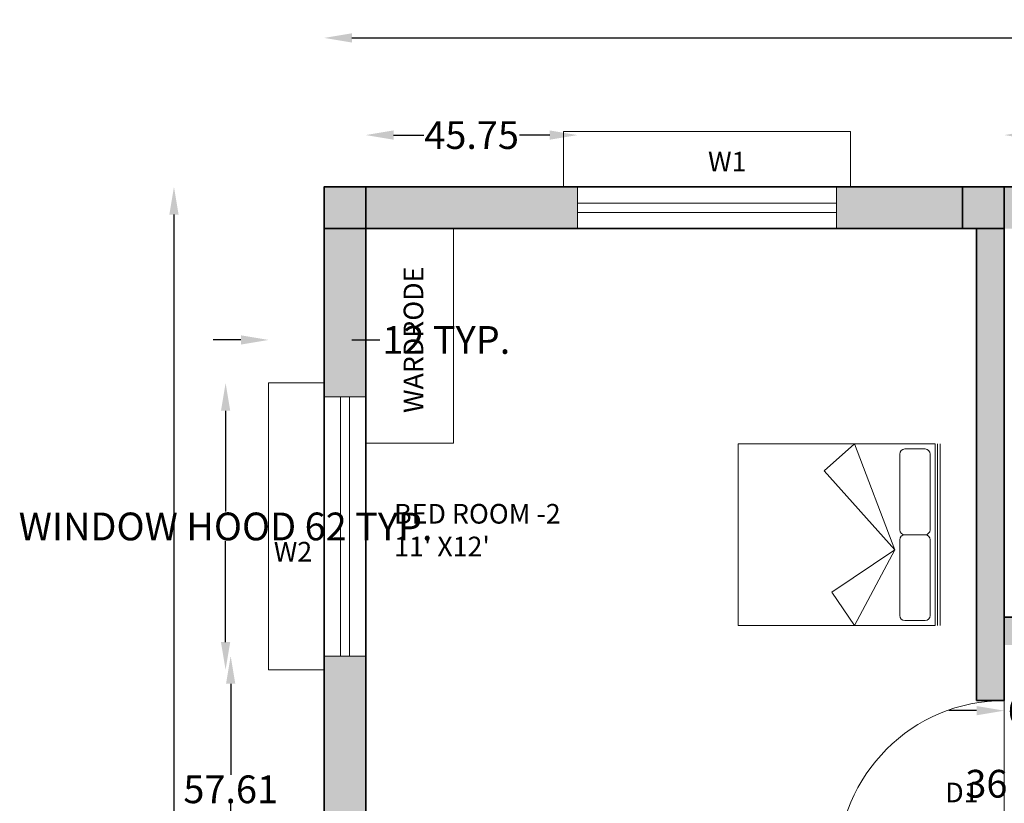
# Model space of a CAD drawing. Units: inches. Extents: x 1994 to 3075, y 3517 to 3950.
# Tile 52 of 58: x 2603 to 2816, y 3781 to 3950. Entities that reach past the tile are written whole.
import ezdxf

# ---------------------------------------------------------------- set-up
doc = ezdxf.new("R2010")
doc.units = ezdxf.units.IN
for name, color, linetype, lineweight in [('A-ANNO-DIMS', 2, 'Continuous', 18), ('A-ANNO-TEXT', 7, 'Continuous', 18), ('A-AREA-IDEN', 7, 'Continuous', 18), ('A-COLS', 7, 'Continuous', 35), ('A-COLS-PATT', 6, 'Continuous', 13), ('A-DOOR', 3, 'Continuous', 18), ('A-FLOR-CASE', 8, 'Continuous', 18), ('A-FURN', 8, 'Continuous', 18), ('A-GLAZ', 4, 'Continuous', 18), ('A-GLAZ-PROJ', 4, 'Continuous', 18), ('A-WALL', 7, 'Continuous', 35), ('A-WALL-PATT', 252, 'Continuous', 13)]:
    doc.layers.add(name, color=color, linetype=linetype, lineweight=lineweight)
doc.styles.get("Standard").update_dxf_attribs({"font": 'arial.ttf'})
doc.dimstyles.get("Standard").update_dxf_attribs({"dimtxt": 6, "dimasz": 6, "dimexe": 0.18, "dimexo": 0.0625, "dimgap": 0.09, "dimtad": 0, "dimtih": 1, "dimtoh": 1, "dimdec": 4, "dimzin": 0, "dimdsep": 46, "dimlunit": 4, "dimtxsty": 'Standard', "dimcen": 0.09, "dimse1": 1, "dimse2": 1, "dimadec": 0, "dimazin": 0, "dimtfac": 1, "dimtdec": 4, "dimtofl": 0, "dimtmove": 0, "dimatfit": 3, "dimfxl": 1, "dimtolj": 1, "dimtzin": 0, "dimarcsym": 0})

# ---------------------------------------------------------------- blocks, each defined once
blk = doc.blocks.new('DOOR-SWING-36IN')
for p, q in [((36, 0), (36, 36)), ((36, 36), (36, 0)), ((0, 3), (36, 3)), ((36, 0), (0, 0)), ((0, 0), (36, 0))]:
    blk.add_line(p, q)
blk.add_arc((36, 0), 36, 90, 180)
blk = doc.blocks.new('BED-DOUBLE-PLAN')
for p, q in [((0, 39.28), (0, 0)), ((0.55, 0), (0.55, 39.28)), ((1.09, 0), (1.09, 39.28)), ((1.09, 39.28), (43.64, 39.28)), ((9.82, 16.37), (18.55, 39.28)), ((25.06, 33.47), (18.55, 39.28)), ((43.64, 39.28), (43.64, 0)), ((2.18, 20.73), (2.18, 37.09)), ((3.27, 38.19), (7.64, 38.19)), ((8.73, 20.73), (8.73, 37.09)), ((9.82, 16.37), (25.06, 33.47)), ((7.64, 19.64), (3.27, 19.64)), ((2.18, 2.18), (2.18, 18.55)), ((8.73, 2.18), (8.73, 18.55)), ((18.55, 0), (9.82, 16.37)), ((23.41, 7.25), (9.82, 16.37)), ((18.55, 0), (23.41, 7.25)), ((7.64, 1.09), (3.27, 1.09)), ((43.64, 0), (1.09, 0))]:
    blk.add_line(p, q)
for centre, start, end in [((3.27, 37.09), 90, 180), ((7.64, 37.09), 0, 90), ((3.27, 20.73), 180, 270), ((3.27, 18.55), 90, 180), ((7.64, 20.73), 270, 0), ((7.64, 18.55), 0, 90), ((3.27, 2.18), 180, 270), ((7.64, 2.18), 270, 0)]:
    blk.add_arc(centre, 1.09, start, end)
blk = doc.blocks.new('WINDOW-56IN-SASH')
for p, q in [((56.01, 9), (0, 9)), ((0, 5.5), (56.01, 5.5)), ((0, 3.5), (56.01, 3.5)), ((0, 0), (56.01, 0))]:
    blk.add_line(p, q)
blk = doc.blocks.new('WINDOW-HOOD-62IN')
for p, q in [((0, 59.01), (0, 62.01)), ((0, 62.01), (12, 62.01)), ((0, 0), (0, 59.01)), ((12, 0), (0, 0))]:
    blk.add_line(p, q)
blk = doc.blocks.new('*D19')
at = {"layer": 'A-ANNO-DIMS', "color": 0, "lineweight": -2, "transparency": 16777216}
for p, q in [((2647.77, 3865.75), (2647.77, 3843.94)), ((2647.77, 3815.74), (2647.77, 3837.55))]:
    blk.add_line(p, q, dxfattribs=at)
at = {"layer": 'A-ANNO-DIMS', "color": 0, "transparency": 16777216}
for points in [[(2646.77, 3865.75), (2648.77, 3865.75), (2647.77, 3871.75)], [(2646.77, 3815.74), (2648.77, 3815.74), (2647.77, 3809.74)]]:
    blk.add_solid(points, dxfattribs=at)
at = {"layer": 'Defpoints', "color": 0, "transparency": 16777216}
for p in [(2647.77, 3871.75), (2657.07, 3871.75), (2657.07, 3809.74)]:
    blk.add_point(p, dxfattribs=at)
at = {"layer": 'A-ANNO-DIMS', "color": 0, "transparency": 16777216, "insert": (2647.77, 3840.74), "char_height": 6, "attachment_point": 5}
blk.add_mtext('\\A1;WINDOW HOOD 62 TYP.', dxfattribs=at)
blk = doc.blocks.new('*D20')
at = {"layer": 'A-ANNO-DIMS', "color": 0, "lineweight": -2, "transparency": 16777216}
for p, q in [((2651.07, 3881.05), (2645.07, 3881.05)), ((2675.07, 3881.05), (2681.07, 3881.05))]:
    blk.add_line(p, q, dxfattribs=at)
at = {"layer": 'A-ANNO-DIMS', "color": 0, "transparency": 16777216}
for points in [[(2651.07, 3882.05), (2651.07, 3880.05), (2657.07, 3881.05)], [(2675.07, 3882.05), (2675.07, 3880.05), (2669.07, 3881.05)]]:
    blk.add_solid(points, dxfattribs=at)
at = {"layer": 'Defpoints', "color": 0, "transparency": 16777216}
for p in [(2669.07, 3881.05), (2657.07, 3871.75), (2669.07, 3871.75)]:
    blk.add_point(p, dxfattribs=at)
at = {"layer": 'A-ANNO-DIMS', "color": 0, "transparency": 16777216, "insert": (2695.48, 3881.05), "char_height": 6, "attachment_point": 5}
blk.add_mtext('\\A1;12 TYP.', dxfattribs=at)
blk = doc.blocks.new('*D22')
at = {"layer": 'A-ANNO-DIMS', "color": 0, "lineweight": -2, "transparency": 16777216}
for p, q in [((2821.47, 3797.13), (2821.47, 3788.28)), ((2821.47, 3773.13), (2821.47, 3781.97))]:
    blk.add_line(p, q, dxfattribs=at)
at = {"layer": 'A-ANNO-DIMS', "color": 0, "transparency": 16777216}
for points in [[(2820.47, 3797.13), (2822.47, 3797.13), (2821.47, 3803.13)], [(2820.47, 3773.13), (2822.47, 3773.13), (2821.47, 3767.13)]]:
    blk.add_solid(points, dxfattribs=at)
at = {"layer": 'Defpoints', "color": 0, "transparency": 16777216}
for p in [(2816.07, 3803.13), (2821.47, 3803.13), (2816.07, 3767.13)]:
    blk.add_point(p, dxfattribs=at)
at = {"layer": 'A-ANNO-DIMS', "color": 0, "transparency": 16777216, "insert": (2821.47, 3785.13), "char_height": 6, "attachment_point": 5}
blk.add_mtext('\\A1;36 TYP.', dxfattribs=at)
blk = doc.blocks.new('*D31')
at = {"layer": 'A-ANNO-DIMS', "color": 0, "lineweight": -2, "transparency": 16777216}
for p, q in [((2675.07, 3946.33), (2844.37, 3946.33)), ((3027.07, 3946.33), (2857.78, 3946.33))]:
    blk.add_line(p, q, dxfattribs=at)
at = {"layer": 'A-ANNO-DIMS', "color": 0, "transparency": 16777216}
for points in [[(2675.07, 3947.33), (2675.07, 3945.33), (2669.07, 3946.33)], [(3027.07, 3947.33), (3027.07, 3945.33), (3033.07, 3946.33)]]:
    blk.add_solid(points, dxfattribs=at)
at = {"layer": 'Defpoints', "color": 0, "transparency": 16777216}
for p in [(3033.07, 3946.33), (2669.07, 3914.13), (3033.07, 3914.13)]:
    blk.add_point(p, dxfattribs=at)
at = {"layer": 'A-ANNO-DIMS', "color": 0, "transparency": 16777216, "insert": (2851.07, 3946.33), "char_height": 6, "attachment_point": 5}
blk.add_mtext('\\A1;364', dxfattribs=at)
blk = doc.blocks.new('*D32')
at = {"layer": 'A-ANNO-DIMS', "color": 0, "lineweight": -2, "transparency": 16777216}
for p, q in [((2636.61, 3908.13), (2636.61, 3730.78)), ((2636.61, 3547.13), (2636.61, 3724.47))]:
    blk.add_line(p, q, dxfattribs=at)
at = {"layer": 'A-ANNO-DIMS', "color": 0, "transparency": 16777216}
for points in [[(2635.61, 3908.13), (2637.61, 3908.13), (2636.61, 3914.13)], [(2635.61, 3547.13), (2637.61, 3547.13), (2636.61, 3541.13)]]:
    blk.add_solid(points, dxfattribs=at)
at = {"layer": 'Defpoints', "color": 0, "transparency": 16777216}
for p in [(2636.61, 3914.13), (2669.07, 3914.13), (2810.07, 3541.13)]:
    blk.add_point(p, dxfattribs=at)
at = {"layer": 'A-ANNO-DIMS', "color": 0, "transparency": 16777216, "insert": (2636.61, 3727.63), "char_height": 6, "attachment_point": 5}
blk.add_mtext('\\A1;373', dxfattribs=at)
blk = doc.blocks.new('*D40')
at = {"layer": 'A-ANNO-DIMS', "color": 0, "lineweight": -2, "transparency": 16777216}
for p, q in [((2684.07, 3925.33), (2690.59, 3925.33)), ((2717.83, 3925.33), (2711.31, 3925.33))]:
    blk.add_line(p, q, dxfattribs=at)
at = {"layer": 'A-ANNO-DIMS', "color": 0, "transparency": 16777216}
for points in [[(2684.07, 3926.33), (2684.07, 3924.33), (2678.07, 3925.33)], [(2717.83, 3926.33), (2717.83, 3924.33), (2723.83, 3925.33)]]:
    blk.add_solid(points, dxfattribs=at)
at = {"layer": 'Defpoints', "color": 0, "transparency": 16777216}
for p in [(2723.83, 3925.33), (2678.07, 3905.13), (2723.83, 3905.13)]:
    blk.add_point(p, dxfattribs=at)
at = {"layer": 'A-ANNO-DIMS', "color": 0, "transparency": 16777216, "insert": (2700.95, 3925.33), "char_height": 6, "attachment_point": 5}
blk.add_mtext('\\A1;45.75', dxfattribs=at)
blk = doc.blocks.new('*D41')
at = {"layer": 'A-ANNO-DIMS', "color": 0, "lineweight": -2, "transparency": 16777216}
for p, q in [((2822.07, 3925.33), (2831.7, 3925.33)), ((2837.7, 3925.33), (2843.7, 3925.33))]:
    blk.add_line(p, q, dxfattribs=at)
at = {"layer": 'A-ANNO-DIMS', "color": 0, "transparency": 16777216}
for points in [[(2822.07, 3926.33), (2822.07, 3924.33), (2816.07, 3925.33)], [(2831.7, 3926.33), (2831.7, 3924.33), (2837.7, 3925.33)]]:
    blk.add_solid(points, dxfattribs=at)
at = {"layer": 'Defpoints', "color": 0, "transparency": 16777216}
for p in [(2837.7, 3925.33), (2816.07, 3905.13), (2837.7, 3905.13)]:
    blk.add_point(p, dxfattribs=at)
at = {"layer": 'A-ANNO-DIMS', "color": 0, "transparency": 16777216, "insert": (2856.29, 3925.33), "char_height": 6, "attachment_point": 5}
blk.add_mtext('\\A1;21.626', dxfattribs=at)
blk = doc.blocks.new('*D44')
at = {"layer": 'A-ANNO-DIMS', "color": 0, "lineweight": -2, "transparency": 16777216}
for p, q in [((2648.87, 3806.74), (2648.87, 3787.09)), ((2648.87, 3761.13), (2648.87, 3780.78))]:
    blk.add_line(p, q, dxfattribs=at)
at = {"layer": 'A-ANNO-DIMS', "color": 0, "transparency": 16777216}
for points in [[(2647.87, 3806.74), (2649.87, 3806.74), (2648.87, 3812.74)], [(2647.87, 3761.13), (2649.87, 3761.13), (2648.87, 3755.13)]]:
    blk.add_solid(points, dxfattribs=at)
at = {"layer": 'Defpoints', "color": 0, "transparency": 16777216}
for p in [(2648.87, 3812.74), (2669.07, 3812.74), (2669.07, 3755.13)]:
    blk.add_point(p, dxfattribs=at)
at = {"layer": 'A-ANNO-DIMS', "color": 0, "transparency": 16777216, "insert": (2648.87, 3783.93), "char_height": 6, "attachment_point": 5}
blk.add_mtext('\\A1;57.61', dxfattribs=at)
blk = doc.blocks.new('*D51')
at = {"layer": 'A-ANNO-DIMS', "color": 0, "lineweight": -2, "transparency": 16777216}
for p, q in [((2810.072038, 3800.926884), (2804.072038, 3800.926884)), ((2828.072038, 3800.926884), (2834.072038, 3800.926884))]:
    blk.add_line(p, q, dxfattribs=at)
at = {"layer": 'A-ANNO-DIMS', "color": 0, "transparency": 16777216}
for points in [[(2810.072038, 3801.926884), (2810.072038, 3799.926884), (2816.072038, 3800.926884)], [(2828.072038, 3801.926884), (2828.072038, 3799.926884), (2822.072038, 3800.926884)]]:
    blk.add_solid(points, dxfattribs=at)
at = {"layer": 'Defpoints', "color": 0, "transparency": 16777216}
for p in [(2816.072038, 3821.126884), (2822.072038, 3821.126884), (2816.072038, 3800.926884)]:
    blk.add_point(p, dxfattribs=at)
at = {"layer": 'A-ANNO-DIMS', "color": 0, "transparency": 16777216, "insert": (2819.072038, 3800.926884), "char_height": 6, "attachment_point": 5}
blk.add_mtext('\\A1;6', dxfattribs=at)

msp = doc.modelspace()

# ---------------------------------------------------------------- hatches: boundary and pattern name
at = {"layer": 'A-COLS-PATT'}
h = msp.add_hatch(color=256, dxfattribs=at)
h.dxf.hatch_style = 1
h.paths.add_polyline_path([(2678.072, 3914.1269), (2669.072, 3914.1269), (2669.072, 3905.1269), (2678.072, 3905.1269)])
h.paths.add_polyline_path([(2816.072, 3914.1269), (2807.072, 3914.1269), (2807.072, 3905.1269), (2816.072, 3905.1269)])
h.paths.add_polyline_path([(2894.9096, 3914.1269), (2885.9096, 3914.1269), (2885.9096, 3905.1269), (2894.9096, 3905.1269)])
h.paths.add_polyline_path([(3033.072, 3914.1269), (3024.072, 3914.1269), (3024.072, 3905.1269), (3033.072, 3905.1269)])
h.paths.add_polyline_path([(3033.072, 3764.1269), (3024.072, 3764.1269), (3024.072, 3755.1269), (3033.072, 3755.1269)])
h.paths.add_polyline_path([(2895.072, 3764.1269), (2886.072, 3764.1269), (2886.072, 3755.1269), (2895.072, 3755.1269)])
h.paths.add_polyline_path([(2816.072, 3764.1269), (2807.072, 3764.1269), (2807.072, 3755.1269), (2816.072, 3755.1269)])
h.paths.add_polyline_path([(2678.072, 3764.1269), (2669.072, 3764.1269), (2669.072, 3755.1269), (2678.072, 3755.1269)])
h.paths.add_polyline_path([(2678.072, 3664.1269), (2669.072, 3664.1269), (2669.072, 3655.1269), (2678.072, 3655.1269)])
h.paths.add_polyline_path([(2816.072, 3664.1269), (2807.072, 3664.1269), (2807.072, 3655.1269), (2816.072, 3655.1269)])
h.paths.add_polyline_path([(3033.072, 3616.1269), (3024.072, 3616.1269), (3024.072, 3607.1269), (3033.072, 3607.1269)])
h.paths.add_polyline_path([(2894.9096, 3616.1269), (2885.9096, 3616.1269), (2885.9096, 3607.1269), (2894.9096, 3607.1269)])
h.paths.add_polyline_path([(2816.072, 3559.1269), (2807.072, 3559.1269), (2807.072, 3550.1269), (2816.072, 3550.1269)])
h.paths.add_polyline_path([(2678.072, 3559.1269), (2669.072, 3559.1269), (2669.072, 3550.1269), (2678.072, 3550.1269)])
at = {"layer": 'A-WALL-PATT'}
h = msp.add_hatch(color=256, dxfattribs=at)
h.dxf.hatch_style = 1
h.paths.add_polyline_path([(2678.072, 3755.1269), (2669.072, 3755.1269), (2669.072, 3718.5523), (2678.072, 3718.5523)])
h.paths.add_polyline_path([(2807.072, 3761.1269), (2678.072, 3761.1269), (2678.072, 3755.1269), (2807.072, 3755.1269)])
h.paths.add_polyline_path([(2678.072, 3812.7371), (2669.072, 3812.7371), (2669.072, 3809.7371), (2669.072, 3764.1269), (2678.072, 3764.1269)])
h.paths.add_polyline_path([(2678.072, 3905.1269), (2669.072, 3905.1269), (2669.072, 3868.7491), (2678.072, 3868.7491)])
h.paths.add_polyline_path([(2723.826, 3914.1269), (2720.826, 3914.1269), (2678.072, 3914.1269), (2678.072, 3905.1269), (2723.826, 3905.1269)])
h.paths.add_polyline_path([(2807.072, 3914.1269), (2779.838, 3914.1269), (2779.838, 3905.1269), (2807.072, 3905.1269)])
h.paths.add_polyline_path([(2837.6979, 3914.1269), (2834.6979, 3914.1269), (2820.9062, 3914.1269), (2816.072, 3914.1269), (2816.072, 3905.1269), (2837.6979, 3905.1269)])
h.paths.add_polyline_path([(2885.9096, 3914.1269), (2869.71, 3914.1269), (2869.71, 3905.1269), (2876.9183, 3905.1269), (2885.9096, 3905.1269)])
h.paths.add_polyline_path([(2933.6904, 3914.1269), (2930.6904, 3914.1269), (2894.9096, 3914.1269), (2894.9096, 3905.1269), (2933.6904, 3905.1269)])
h.paths.add_polyline_path([(3024.072, 3914.1269), (2989.7025, 3914.1269), (2989.7025, 3905.1269), (3024.072, 3905.1269)])
h.paths.add_polyline_path([(3033.072, 3905.1269), (3024.072, 3905.1269), (3024.072, 3861.4192), (3033.072, 3861.4192)])
h.paths.add_polyline_path([(3033.072, 3805.4072), (3024.072, 3805.4072), (3024.072, 3764.1269), (3033.072, 3764.1269)])
h.paths.add_polyline_path([(3033.072, 3755.1269), (3024.072, 3755.1269), (3024.072, 3732.1247), (3033.072, 3732.1247), (3033.072, 3735.1247)])
h.paths.add_polyline_path([(3024.072, 3761.1269), (2895.072, 3761.1269), (2895.072, 3755.1269), (3024.072, 3755.1269)])
h.paths.add_polyline_path([(3033.072, 3676.1126), (3024.072, 3676.1126), (3024.072, 3616.1269), (3033.072, 3616.1269)])
h.paths.add_polyline_path([(3024.072, 3613.1269), (2959.4908, 3613.1269), (2959.4908, 3607.1269), (3024.072, 3607.1269)])
h.paths.add_polyline_path([(2914.1254, 3613.1269), (2894.9096, 3613.1269), (2894.9096, 3607.1269), (2914.1254, 3607.1269)])
h.paths.add_polyline_path([(2885.9096, 3613.1269), (2852.072, 3613.1269), (2852.072, 3607.1269), (2885.9096, 3607.1269)])
h.paths.add_polyline_path([(2822.072, 3613.1269), (2810.072, 3613.1269), (2810.072, 3559.1269), (2816.072, 3559.1269), (2816.072, 3607.1269), (2822.072, 3607.1269)])
h.paths.add_polyline_path([(2933.072, 3607.1269), (2924.072, 3607.1269), (2924.072, 3550.1269), (2892.072, 3550.1269), (2816.072, 3550.1269), (2810.072, 3550.1269), (2810.072, 3541.1269), (2892.072, 3541.1269), (2933.072, 3541.1269)])
h.paths.add_polyline_path([(2807.072, 3559.1269), (2678.072, 3559.1269), (2678.072, 3550.1269), (2807.072, 3550.1269)])
h.paths.add_polyline_path([(2678.072, 3655.1269), (2669.072, 3655.1269), (2669.072, 3559.1269), (2678.072, 3559.1269)])
h.paths.add_polyline_path([(2678.072, 3686.5403), (2669.072, 3686.5403), (2669.072, 3664.1269), (2678.072, 3664.1269)])
h.paths.add_polyline_path([(2807.072, 3661.1269), (2678.072, 3661.1269), (2678.072, 3655.1269), (2807.072, 3655.1269)])
h.paths.add_polyline_path([(2816.072, 3755.1269), (2810.072, 3755.1269), (2810.072, 3703.1269), (2816.072, 3703.1269)])
h.paths.add_polyline_path([(2816.072, 3905.1269), (2810.072, 3905.1269), (2810.072, 3803.1269), (2816.072, 3803.1269), (2816.072, 3815.1269)])
h.paths.add_polyline_path([(2886.072, 3821.1269), (2852.072, 3821.1269), (2852.072, 3815.1269), (2886.072, 3815.1269)])
h.paths.add_polyline_path([(2822.072, 3821.1269), (2816.072, 3821.1269), (2816.072, 3815.1269), (2822.072, 3815.1269)])
h.paths.add_polyline_path([(2892.072, 3905.1269), (2886.072, 3905.1269), (2886.072, 3803.1269), (2892.072, 3803.1269)])

# ---------------------------------------------------------------- linework, layer by layer
at = {"layer": 'A-COLS'}
for points in [[(2669.072, 3905.1269), (2678.072, 3905.1269), (2678.072, 3914.1269), (2669.072, 3914.1269)], [(2807.072, 3905.1269), (2816.072, 3905.1269), (2816.072, 3914.1269), (2807.072, 3914.1269)]]:
    msp.add_lwpolyline(points, close=True, dxfattribs=at)
at = {"layer": 'A-FLOR-CASE'}
for p, q in [((2697.016, 3905.1269), (2697.016, 3858.7564)), ((2697.016, 3858.7564), (2678.072, 3858.7564))]:
    msp.add_line(p, q, dxfattribs=at)
at = {"layer": 'A-GLAZ'}
for p, q in [((2723.826, 3914.1269), (2723.826, 3905.1269)), ((2779.838, 3905.1269), (2779.838, 3914.1269)), ((2678.072, 3868.7491), (2669.072, 3868.7491)), ((2669.072, 3812.7371), (2678.072, 3812.7371))]:
    msp.add_line(p, q, dxfattribs=at)
at = {"layer": 'A-GLAZ-PROJ'}
for p, q in [((2723.826, 3914.1269), (2720.826, 3914.1269)), ((2669.072, 3812.7371), (2669.072, 3809.7371))]:
    msp.add_line(p, q, dxfattribs=at)
at = {"layer": 'A-WALL'}
for p, q in [((2669.072, 3914.1269), (2669.072, 3550.1269)), ((2669.072, 3914.1269), (3033.072, 3914.1269)), ((2678.072, 3905.1269), (2678.072, 3761.1269)), ((2678.072, 3905.1269), (2810.072, 3905.1269)), ((2810.072, 3905.1269), (2810.072, 3803.1269)), ((2816.072, 3905.1269), (2816.072, 3803.1269)), ((2816.072, 3821.1269), (2822.072, 3821.1269)), ((2816.072, 3815.1269), (2816.072, 3803.1269)), ((2816.072, 3803.1269), (2810.072, 3803.1269))]:
    msp.add_line(p, q, dxfattribs=at)

# ---------------------------------------------------------------- block references
at = {"layer": 'A-DOOR'}
msp.add_blockref('DOOR-SWING-36IN', (2780.072, 3767.127), dxfattribs=at)
at = {"layer": 'A-FURN', "extrusion": (0, 0, -1), "zscale": -1}
msp.add_blockref('BED-DOUBLE-PLAN', (-2802.2121, 3819.3), dxfattribs=at)
at = {"layer": 'A-GLAZ'}
msp.add_blockref('WINDOW-56IN-SASH', (2723.826, 3905.127), dxfattribs=at)
at = {"layer": 'A-GLAZ', "rotation": 89.9999999999985}
msp.add_blockref('WINDOW-56IN-SASH', (2678.0719, 3812.7371), dxfattribs=at)
at = {"layer": 'A-GLAZ-PROJ', "rotation": 269.9999999999988}
msp.add_blockref('WINDOW-HOOD-62IN', (2720.8259, 3926.1269), dxfattribs=at)
at = {"layer": 'A-GLAZ-PROJ'}
msp.add_blockref('WINDOW-HOOD-62IN', (2657.072, 3809.737), dxfattribs=at)

# ---------------------------------------------------------------- texts
at = {"layer": 'A-ANNO-TEXT', "char_height": 4.24528, "attachment_point": 1}
for s, insert in [('W1', (2752.0433, 3921.7054)), ('W2', (2658.1859, 3837.4033)), ('D1', (2803.3066, 3785.3592))]:
    msp.add_mtext_dynamic_manual_height_columns(s, width=102.693633, gutter_width=21.2264, heights=[0], dxfattribs=dict(at, insert=insert))
at = {"layer": 'A-ANNO-TEXT', "insert": (2686.2541, 3865.259), "char_height": 4.24528, "attachment_point": 1, "rotation": 90}
msp.add_mtext_dynamic_manual_height_columns('WARDRODE', width=102.693633, gutter_width=21.2264, heights=[0], dxfattribs=at)
at = {"layer": 'A-AREA-IDEN', "insert": (2684.1917, 3845.603), "char_height": 4.245283, "attachment_point": 1}
msp.add_mtext_dynamic_manual_height_columns("BED ROOM -2\\P11' X12'", width=102.693633, gutter_width=21.2264, heights=[0], dxfattribs=at)

# ---------------------------------------------------------------- dimensions: what is measured, and where the dimension line sits
at = {"layer": 'A-ANNO-DIMS'}
for base, p1, p2, override, picture, middle in [((3033.072, 3946.3269), (2669.072, 3914.1269), (3033.072, 3914.1269), {"dimdec": 0, "dimlfac": 1, "dimrnd": 0, "dimzin": 0, "dimdsep": 46, "dimlunit": 2}, '*D31', (2851.072, 3946.3269)), ((2723.826, 3925.3269), (2678.072, 3905.1269), (2723.826, 3905.1269), {"dimdec": 2, "dimlfac": 1, "dimrnd": 0, "dimzin": 0, "dimdsep": 46, "dimlunit": 2}, '*D40', (2700.949, 3925.3269)), ((2837.6979, 3925.3269), (2816.072, 3905.1269), (2837.6979, 3905.1269), {"dimdec": 3, "dimlfac": 1, "dimrnd": 0, "dimzin": 0, "dimdsep": 46, "dimlunit": 2}, '*D41', (2856.2913, 3925.3269))]:
    dim = msp.add_linear_dim(base=base, p1=p1, p2=p2, dimstyle='Standard', override=override, dxfattribs=at)
    dim.commit()
    dim.dimension.update_dxf_attribs({"geometry": picture, "text_midpoint": middle})
for base, p1, p2, angle, override, picture, middle in [((2636.6096, 3914.1269), (2810.072, 3541.1269), (2669.072, 3914.1269), 90, {"dimdec": 0, "dimlfac": 1, "dimrnd": 0, "dimzin": 0, "dimdsep": 46, "dimlunit": 2}, '*D32', (2636.6096, 3727.6269)), ((2816.072, 3800.9269), (2822.072, 3821.1269), (2816.072, 3821.1269), 180, {"dimdec": 0, "dimlfac": 1, "dimrnd": 0, "dimzin": 0, "dimdsep": 46, "dimlunit": 2}, '*D51', (2819.072, 3800.9269)), ((2648.872, 3812.7371), (2669.072, 3755.1269), (2669.072, 3812.7371), 90, {"dimdec": 2, "dimlfac": 1, "dimrnd": 0, "dimzin": 0, "dimdsep": 46, "dimlunit": 2}, '*D44', (2648.872, 3783.932))]:
    dim = msp.add_linear_dim(base=base, p1=p1, p2=p2, angle=angle, dimstyle='Standard', override=override, dxfattribs=at)
    dim.commit()
    dim.dimension.update_dxf_attribs({"geometry": picture, "text_midpoint": middle})
dim = msp.add_linear_dim(base=(2669.072, 3881.0509), p1=(2657.072, 3871.7491), p2=(2669.072, 3871.7491), text='<> TYP.', dimstyle='Standard', override={"dimdec": 0, "dimlfac": 1, "dimrnd": 0, "dimzin": 0, "dimdsep": 46, "dimlunit": 2}, dxfattribs=at)
dim.commit()
dim.dimension.update_dxf_attribs({"geometry": '*D20', "text_midpoint": (2695.4826, 3881.0509)})
for base, p1, p2, text, picture, middle in [((2647.7702, 3871.7491), (2657.072, 3809.7371), (2657.072, 3871.7491), 'WINDOW HOOD <> TYP.', '*D19', (2647.7702, 3840.7431)), ((2821.472, 3803.1269), (2816.072, 3767.1269), (2816.072, 3803.1269), '<> TYP.', '*D22', (2821.472, 3785.1269))]:
    dim = msp.add_linear_dim(base=base, p1=p1, p2=p2, angle=90, text=text, dimstyle='Standard', override={"dimdec": 0, "dimlfac": 1, "dimrnd": 0, "dimzin": 0, "dimdsep": 46, "dimlunit": 2}, dxfattribs=at)
    dim.commit()
    dim.dimension.update_dxf_attribs({"geometry": picture, "text_midpoint": middle})

doc.saveas('drawing.dxf')
